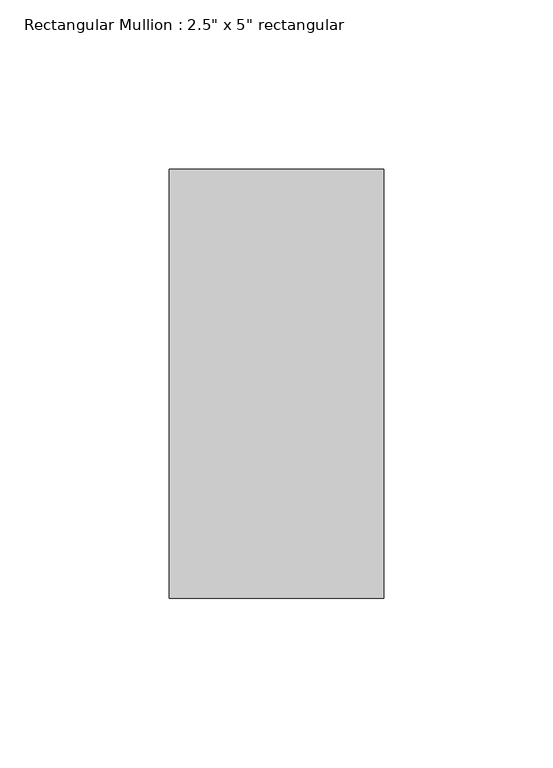
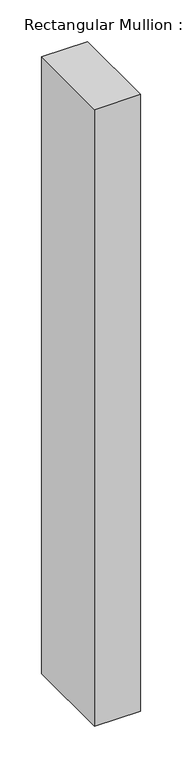
"""IFC4 building model written with IfcOpenShell, lengths in millimetres: member geometry."""

from ifc_helpers import new_model, si_unit, frame, origin, place, context, project, spatial, polyline, outline, extrude, source, transform, mapped, element, save


def member_8719ea0b(model_context):
    return source(origin(), model_context, "Body", "SweptSolid", [
        extrude(outline(polyline([(0.0, 63.5), (0.0, -63.5), (-63.5, -63.5), (-63.5, 63.5), (0.0, 63.5)])), frame((0.0, 0.0, -902.5301773), z_axis=(0.0, 0.0, 1.0), x_axis=(1.0, 0.0, 0.0)), (0.0, 0.0, 1.0), 902.5301773),
    ])


if __name__ == "__main__":
    model = new_model("IFC4")
    model_context = context("Model", 3, world=origin())
    ifc_project = project(units=[si_unit("LENGTHUNIT", "METRE", prefix="MILLI")], contexts=[model_context])
    site = spatial("IfcSite", under=ifc_project)
    building = spatial("IfcBuilding", under=site)
    placement = place(None, origin())
    member_shape = member_8719ea0b(model_context)
    element("IfcMember", 1, ObjectType="Rectangular Mullion : 2.5\" x 5\" rectangular", at=placement, inside=building, context=model_context, shape_type="MappedRepresentation", body=[
        mapped(member_shape, transform((0.0, 0.0, 0.0), x_axis=(1.0, 0.0, 0.0), y_axis=(0.0, 1.0, 0.0), z_axis=(0.0, 0.0, 1.0))),
    ])
    save(model, "model.ifc")

# Revit data of these elements
# Type "Rectangular Mullion : 2.5\" x 5\" rectangular"
#   built-in parameter 1007304 = 0.416667 (stored number, unit not read)
#   built-in parameter 1007301 = 0.104167 (stored number, unit not read)
#   built-in parameter 1007300 = 0.104167 (stored number, unit not read)
# Element 1 (IfcMember, "Rectangular Mullion : 2.5\" x 5\" rectangular")
#   Materials on its faces: "Aluminum"
# Materials
#   "Aluminum": class "Metal", colour RGB 247 247 247, transparency 0, Description = "Aluminum 6061", Cost = 0
